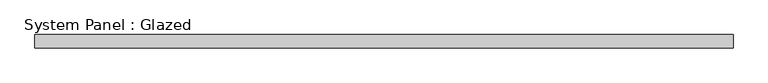
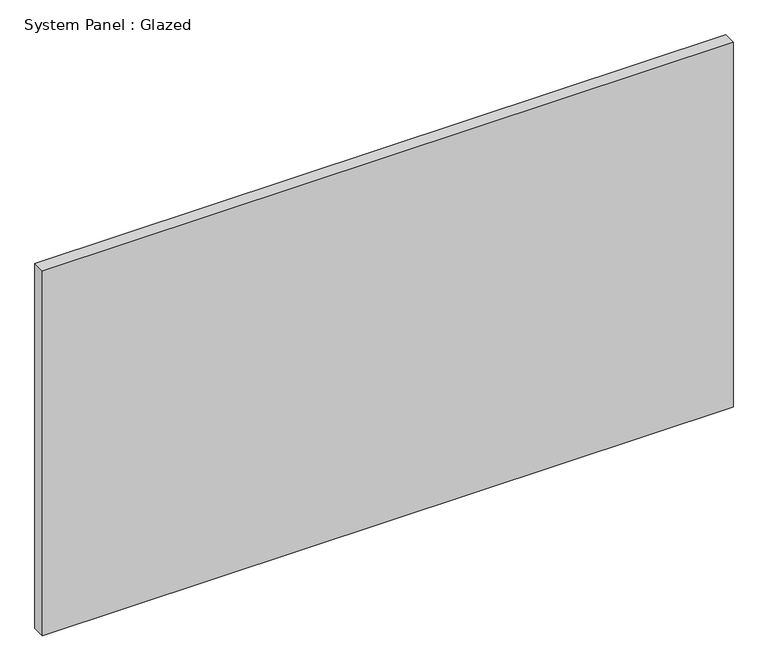
"""IFC4 building model written with IfcOpenShell, lengths in millimetres: plate geometry, System Panel : Glazed."""

from ifc_helpers import new_model, si_unit, origin, origin_with_axes, place, context, project, spatial, polyline, outline, extrude, source, transform, mapped, element, save


def system_panel_glazed_e6893c60(model_context):
    return source(origin(), model_context, "Body", "SweptSolid", [
        extrude(outline(polyline([(659.1499998, 24.5), (-659.1499998, 24.5), (-659.1499998, 49.5), (659.1499998, 49.5), (659.1499998, 24.5)])), origin_with_axes(), (0.0, 0.0, 1.0), 736.6),
    ])


if __name__ == "__main__":
    model = new_model("IFC4")
    model_context = context("Model", 3, world=origin())
    ifc_project = project(units=[si_unit("LENGTHUNIT", "METRE", prefix="MILLI")], contexts=[model_context])
    site = spatial("IfcSite", under=ifc_project)
    building = spatial("IfcBuilding", under=site)
    placement = place(None, origin())
    system_panel_glazed_shape = system_panel_glazed_e6893c60(model_context)
    element("IfcPlate", 1, ObjectType="System Panel : Glazed", at=placement, inside=building, context=model_context, shape_type="MappedRepresentation", body=[
        mapped(system_panel_glazed_shape, transform((0.0, 0.0, 0.0), x_axis=(1.0, 0.0, 0.0), y_axis=(0.0, 1.0, 0.0), z_axis=(0.0, 0.0, 1.0))),
    ])
    save(model, "model.ifc")

# Revit data of these elements
# Type "System Panel : Glazed"
#   Keynote = "H11"
#   Construction Type Id = "GSP4R"
#   Analytic Construction = "1/8 in Pilkington single glazing"
#   Visual Light Transmittance = 0.9
#   Solar Heat Gain Coefficient = 0.86
#   Heat Transfer Coefficient (U) = 6.7069 W/(m²·K)
#   Define Thermal Properties by = 1
# Element 1 (IfcPlate, "System Panel : Glazed")
#   Materials on its faces: "Glass"
# Materials
#   "Glass": class "Glass", colour RGB 0 128 192, transparency 0.9, Description = "Soda Lime Glass", Cost = 0
